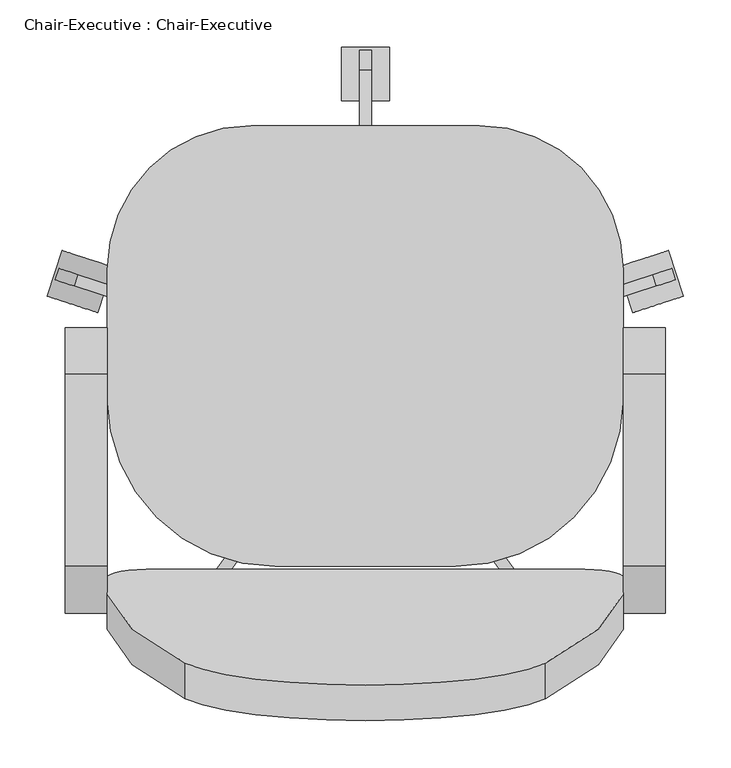
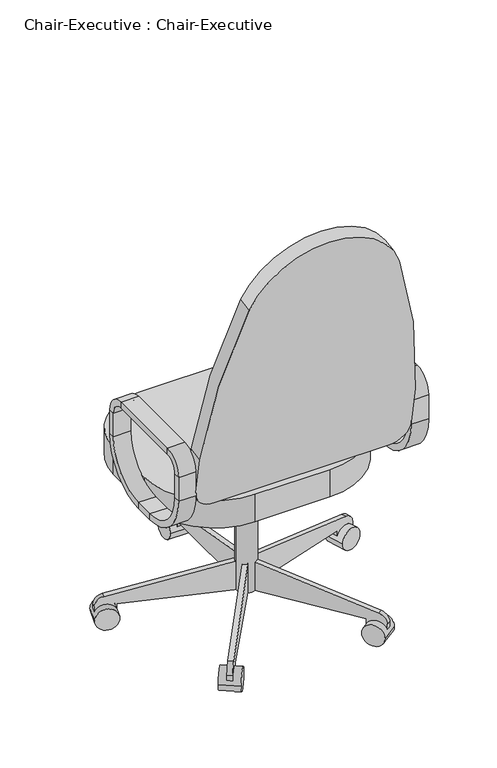
"""IFC4 building model written with IfcOpenShell, lengths in millimetres: furniture geometry, Chair-Executive : Chair-Executive."""

from ifc_helpers import new_model, si_unit, point, frame, frame_2d, origin, place, context, project, spatial, polyline, circle_curve, trimmed, segment, composite_curve, outline, extrude, source, transform, mapped, element, save
from ifc_brep_helpers import plane_surface, cylinder_surface, revolved_surface, advanced_brep


def chair_executive_chair_executive_a6d00652(model_context):
    return source(origin(), model_context, "Body", "SolidModel", [
        extrude(outline(polyline([(69.7459016, 383.7835944), (69.7459016, 371.0835944), (18.9459016, 283.0954134), (-19.1540984, 283.0954134), (-19.1540984, 383.7835944), (69.7459016, 383.7835944)])), frame((90.1908197, 0.0, 0.0), z_axis=(1.0, 0.0, 0.0), x_axis=(0.0, 1.0, 0.0)), (0.0, 0.0, 1.0), 101.6),
        extrude(outline(composite_curve([segment(polyline([(311.0459016, 53.5835944), (18.9459016, 53.5835944), (18.9459016, 129.7835944), (44.3459016, 129.7835944), (340.8565654, 77.5007643)]), True, "CONTINUOUS"), segment(trimmed(circle_curve(frame_2d((336.4459016, 52.4866474)), 25.4), [point((340.8565654, 77.5007643))], [point((361.8459016, 52.4866474))], False, "CARTESIAN"), True, "CONTINUOUS"), segment(polyline([(361.8459016, 52.4866474), (361.8459016, 28.1835944), (311.0459016, 28.1835944), (311.0459016, 53.5835944)]), True, "CONTINUOUS")], self_intersect=False)), frame((134.6408197, 0.0, 0.0), z_axis=(1.0, 0.0, 0.0), x_axis=(0.0, 1.0, 0.0)), (0.0, 0.0, 1.0), 12.7),
        extrude(outline(composite_curve([segment(trimmed(circle_curve(frame_2d((336.4459016, 28.1835944)), 28.2002727), [point((308.2456289, 28.1835944))], [point((364.6461744, 28.1835944))], False, "CARTESIAN"), True, "CONTINUOUS"), segment(trimmed(circle_curve(frame_2d((336.4459016, 28.1835944)), 28.2002727), [point((364.6461744, 28.1835944))], [point((308.2456289, 28.1835944))], False, "CARTESIAN"), True, "CONTINUOUS")], self_intersect=False)), frame((115.5908197, 0.0, 0.0), z_axis=(1.0, 0.0, 0.0), x_axis=(0.0, 1.0, 0.0)), (0.0, 0.0, 1.0), 50.8),
        extrude(outline(composite_curve([segment(polyline([(25.4, 0.0), (25.4, 292.1000001), (101.6, 292.1000001), (101.6, 266.7), (49.3171699, -29.8106636)]), True, "CONTINUOUS"), segment(trimmed(circle_curve(frame_2d((24.303053, -25.4)), 25.4), [point((49.3171699, -29.8106636))], [point((24.303053, -50.8))], False, "CARTESIAN"), True, "CONTINUOUS"), segment(polyline([(24.303053, -50.8), (0.0, -50.8), (0.0, 0.0), (25.4, 0.0)]), True, "CONTINUOUS")], self_intersect=False)), frame((-138.7750467, 103.1705568, 28.1835944), z_axis=(0.3090169943749487, 0.9510565162951532, 0.0), x_axis=(0.0, 0.0, 1.0)), (0.0, 0.0, 1.0), 12.7),
        extrude(outline(composite_curve([segment(trimmed(circle_curve(frame_2d((0.0, -28.2002727)), 28.2002727), [point((0.0, -56.4005454))], [point((0.0, 0.0))], False, "CARTESIAN"), True, "CONTINUOUS"), segment(trimmed(circle_curve(frame_2d((0.0, -28.2002727)), 28.2002727), [point((0.0, 0.0))], [point((0.0, -56.4005454))], False, "CARTESIAN"), True, "CONTINUOUS")], self_intersect=False)), frame((-195.638709, 101.6163254, 28.1835944), z_axis=(0.3090169943749487, 0.9510565162951532, 0.0), x_axis=(0.0, 0.0, -1.0)), (0.0, 0.0, 1.0), 50.8),
        extrude(outline(composite_curve([segment(polyline([(25.4, 0.0), (25.4, 292.1), (101.6, 292.1), (101.6, 266.7), (49.3171699, -29.8106637)]), True, "CONTINUOUS"), segment(trimmed(circle_curve(frame_2d((24.303053, -25.3999999)), 25.4), [point((49.3171699, -29.8106637))], [point((24.303053, -50.8))], False, "CARTESIAN"), True, "CONTINUOUS"), segment(polyline([(24.303053, -50.8), (0.0, -50.8), (0.0, 0.0), (25.4, 0.0)]), True, "CONTINUOUS")], self_intersect=False)), frame((-25.5639946, -221.1003988, 28.1835944), z_axis=(-0.8090169943749459, 0.5877852522924754, 0.0), x_axis=(0.0, 0.0, 1.0)), (0.0, 0.0, 1.0), 12.7),
        extrude(outline(composite_curve([segment(trimmed(circle_curve(frame_2d((0.0, -28.2002727)), 28.2002727), [point((0.0, -56.4005455))], [point((0.0, 0.0))], False, "CARTESIAN"), True, "CONTINUOUS"), segment(trimmed(circle_curve(frame_2d((0.0, -28.2002727)), 28.2002727), [point((0.0, 0.0))], [point((0.0, -56.4005455))], False, "CARTESIAN"), True, "CONTINUOUS")], self_intersect=False)), frame((-41.6576707, -275.6612394, 28.1835944), z_axis=(-0.8090169943749458, 0.5877852522924754, 0.0), x_axis=(0.0, 0.0, -1.0)), (0.0, 0.0, 1.0), 50.8),
        extrude(outline(composite_curve([segment(polyline([(-25.4, 0.0), (0.0, 0.0), (0.0, -50.8), (-24.303053, -50.8)]), True, "CONTINUOUS"), segment(trimmed(circle_curve(frame_2d((-24.303053, -25.3999999)), 25.4), [point((-24.303053, -50.8))], [point((-49.3171699, -29.8106636))], False, "CARTESIAN"), True, "CONTINUOUS"), segment(polyline([(-49.3171699, -29.8106636), (-101.6, 266.7), (-101.6, 292.1), (-25.4, 292.1), (-25.4, 0.0)]), True, "CONTINUOUS")], self_intersect=False)), frame((307.545634, -221.1003988, 28.1835944), z_axis=(0.8090169943749499, 0.5877852522924699, 0.0), x_axis=(0.0, 0.0, -1.0)), (0.0, 0.0, 1.0), 12.7),
        extrude(outline(composite_curve([segment(trimmed(circle_curve(frame_2d((0.0, -28.2002727)), 28.2002727), [point((0.0, -56.4005455))], [point((0.0, 0.0))], False, "CARTESIAN"), True, "CONTINUOUS"), segment(trimmed(circle_curve(frame_2d((0.0, -28.2002727)), 28.2002727), [point((0.0, 0.0))], [point((0.0, -56.4005455))], False, "CARTESIAN"), True, "CONTINUOUS")], self_intersect=False)), frame((323.63931, -275.6612394, 28.1835944), z_axis=(0.8090169943749499, 0.5877852522924699, 0.0), x_axis=(0.0, 0.0, 1.0)), (0.0, 0.0, 1.0), 50.8),
        extrude(outline(composite_curve([segment(polyline([(-25.4, 0.0), (0.0, 0.0), (0.0, -50.8), (-24.303053, -50.8)]), True, "CONTINUOUS"), segment(trimmed(circle_curve(frame_2d((-24.303053, -25.4)), 25.4), [point((-24.303053, -50.8))], [point((-49.3171699, -29.8106637))], False, "CARTESIAN"), True, "CONTINUOUS"), segment(polyline([(-49.3171699, -29.8106637), (-101.6, 266.7), (-101.6, 292.1), (-25.4, 292.1), (-25.4, 0.0)]), True, "CONTINUOUS")], self_intersect=False)), frame((420.756686, 103.1705568, 28.1835944), z_axis=(-0.3090169943749423, 0.9510565162951553, 0.0), x_axis=(0.0, 0.0, -1.0)), (0.0, 0.0, 1.0), 12.7),
        extrude(outline(composite_curve([segment(trimmed(circle_curve(frame_2d((0.0, -28.2002727)), 28.2002727), [point((0.0, -56.4005455))], [point((0.0, 0.0))], False, "CARTESIAN"), True, "CONTINUOUS"), segment(trimmed(circle_curve(frame_2d((0.0, -28.2002727)), 28.2002727), [point((0.0, 0.0))], [point((0.0, -56.4005455))], False, "CARTESIAN"), True, "CONTINUOUS")], self_intersect=False)), frame((477.6203484, 101.6163254, 28.1835944), z_axis=(-0.3090169943749423, 0.9510565162951553, 0.0), x_axis=(0.0, 0.0, 1.0)), (0.0, 0.0, 1.0), 50.8),
        extrude(outline(composite_curve([segment(trimmed(circle_curve(frame_2d((140.9908197, 18.9459016)), 25.4), [point((115.5908197, 18.9459016))], [point((166.3908197, 18.9459016))], False, "CARTESIAN"), True, "CONTINUOUS"), segment(trimmed(circle_curve(frame_2d((140.9908197, 18.9459016)), 25.4), [point((166.3908197, 18.9459016))], [point((115.5908197, 18.9459016))], False, "CARTESIAN"), True, "CONTINUOUS")], self_intersect=False)), frame((0.0, 0.0, 53.5835944), z_axis=(0.0, 0.0, 1.0), x_axis=(1.0, 0.0, 0.0)), (0.0, 0.0, 1.0), 330.5914056),
        extrude(outline(composite_curve([segment(trimmed(circle_curve(frame_2d((20.3408197, 129.4961016)), 152.4), [point((-132.0591803, 129.4961016))], [point((20.3408197, 281.8961016))], False, "CARTESIAN"), True, "CONTINUOUS"), segment(polyline([(20.3408197, 281.8961016), (261.6408197, 281.8961016)]), True, "CONTINUOUS"), segment(trimmed(circle_curve(frame_2d((261.6408197, 129.4961016)), 152.4), [point((261.6408197, 281.8961016))], [point((414.0408197, 129.4961016))], False, "CARTESIAN"), True, "CONTINUOUS"), segment(polyline([(414.0408197, 129.4961016), (414.0408197, -6.4540984)]), True, "CONTINUOUS"), segment(trimmed(circle_curve(frame_2d((236.2408197, -6.4540984)), 177.8), [point((414.0408197, -6.4540984))], [point((236.2408197, -184.2540984))], False, "CARTESIAN"), True, "CONTINUOUS"), segment(polyline([(236.2408197, -184.2540984), (45.7408197, -184.2540984)]), True, "CONTINUOUS"), segment(trimmed(circle_curve(frame_2d((45.7408197, -6.4540984)), 177.8), [point((45.7408197, -184.2540984))], [point((-132.0591803, -6.4540984))], False, "CARTESIAN"), True, "CONTINUOUS"), segment(polyline([(-132.0591803, -6.4540984), (-132.0591803, 129.4961016)]), True, "CONTINUOUS")], self_intersect=False)), frame((0.0, 0.0, 383.7835944), z_axis=(0.0, 0.0, 1.0), x_axis=(1.0, 0.0, 0.0)), (0.0, 0.0, 1.0), 73.4164056),
        extrude(outline(composite_curve([segment(trimmed(circle_curve(frame_2d((0.0, -50.8)), 50.8), [point((0.0, 0.0))], [point((50.8, -50.8))], False, "CARTESIAN"), True, "CONTINUOUS"), segment(polyline([(50.8, -50.8), (50.8, -152.4)]), True, "CONTINUOUS"), segment(trimmed(circle_curve(frame_2d((-1471.2021854, -74.3913617)), 1524.0), [point((50.8, -152.4))], [point((-31.75, -574.9444618))], False, "CARTESIAN"), True, "CONTINUOUS"), segment(trimmed(circle_curve(frame_2d((-222.25, -504.2338544)), 203.2), [point((-31.75, -574.9444618))], [point((-412.75, -574.9444618))], False, "CARTESIAN"), True, "CONTINUOUS"), segment(trimmed(circle_curve(frame_2d((1026.7021854, -74.3913617)), 1524.0), [point((-412.75, -574.9444618))], [point((-495.3, -152.4))], False, "CARTESIAN"), True, "CONTINUOUS"), segment(polyline([(-495.3, -152.4), (-495.3, -50.8)]), True, "CONTINUOUS"), segment(trimmed(circle_curve(frame_2d((-444.5, -50.8)), 50.8), [point((-495.3, -50.8))], [point((-444.5, 0.0))], False, "CARTESIAN"), True, "CONTINUOUS"), segment(polyline([(-444.5, 0.0), (0.0, 0.0)]), True, "CONTINUOUS")], self_intersect=False)), frame((363.2408197, -224.5698964, 503.1641822), z_axis=(0.0, 0.9848077530122084, 0.17364817766692853), x_axis=(1.0, 0.0, 0.0)), (0.0, 0.0, 1.0), 38.1),
        advanced_brep(
        [(414.0408197, -233.6623012, 546.1), (414.0408197, -108.0540984, 420.4917972), (458.4908197, -108.0540984, 420.4917972), (458.4908197, -233.6623012, 546.1), (414.0408197, -217.7873012, 546.1), (414.0408197, -108.0540984, 436.3667972), (458.4908197, -217.7873012, 546.1), (458.4908197, -108.0540984, 436.3667972), (458.4908197, -233.6623012, 609.6), (414.0408197, -233.6623012, 609.6), (414.0408197, -217.7873012, 609.6), (458.4908197, -217.7873012, 609.6), (414.0408197, -184.2540984, 659.0082028), (458.4908197, -184.2540984, 659.0082028), (414.0408197, -184.2540984, 643.1332028), (458.4908197, -184.2540984, 643.1332028), (458.4908197, 18.9459016, 659.0082028), (414.0408197, 18.9459016, 659.0082028), (414.0408197, 18.9459016, 643.1332028), (458.4908197, 18.9459016, 643.1332028), (414.0408197, 68.3541044, 609.6), (458.4908197, 68.3541044, 609.6), (414.0408197, 52.4791044, 609.6), (458.4908197, 52.4791044, 609.6), (458.4908197, 68.3541044, 546.1), (414.0408197, 68.3541044, 546.1), (414.0408197, 52.4791044, 546.1), (458.4908197, 52.4791044, 546.1), (414.0408197, -57.2540984, 420.4917972), (458.4908197, -57.2540984, 420.4917972), (414.0408197, -57.2540984, 436.3667972), (458.4908197, -57.2540984, 436.3667972)],
        [
            (0, 1, circle_curve(frame((414.0408197, -108.0540984, 546.1), z_axis=(1.0, 0.0, 0.0), x_axis=(0.0, 0.0, -1.0)), 125.6082028)),
            (1, 2),
            (2, 3, circle_curve(frame((458.4908197, -108.0540984, 546.1), z_axis=(-1.0, 0.0, 0.0), x_axis=(0.0, 0.0, -1.0)), 125.6082028)),
            (3, 0),
            (4, 5, circle_curve(frame((414.0408197, -108.0540984, 546.1), z_axis=(1.0, 0.0, 0.0), x_axis=(0.0, 0.0, -1.0)), 109.7332028)),
            (5, 1),
            (0, 4),
            (6, 7, circle_curve(frame((458.4908197, -108.0540984, 546.1), z_axis=(1.0, 0.0, 0.0), x_axis=(0.0, 0.0, -1.0)), 109.7332028)),
            (7, 5),
            (4, 6),
            (2, 7),
            (6, 3),
            (3, 8),
            (8, 9),
            (9, 0),
            (9, 10),
            (10, 4),
            (10, 11),
            (11, 6),
            (11, 8),
            (12, 9, circle_curve(frame((414.0408197, -184.2540984, 609.6), z_axis=(1.0, 0.0, 0.0), x_axis=(0.0, -1.0, 0.0)), 49.4082028)),
            (8, 13, circle_curve(frame((458.4908197, -184.2540984, 609.6), z_axis=(-1.0, 0.0, 0.0), x_axis=(0.0, -1.0, 0.0)), 49.4082028)),
            (13, 12),
            (14, 10, circle_curve(frame((414.0408197, -184.2540984, 609.6), z_axis=(1.0, 0.0, 0.0), x_axis=(0.0, -1.0, 0.0)), 33.5332028)),
            (12, 14),
            (15, 11, circle_curve(frame((458.4908197, -184.2540984, 609.6), z_axis=(1.0, 0.0, 0.0), x_axis=(0.0, -1.0, 0.0)), 33.5332028)),
            (14, 15),
            (15, 13),
            (13, 16),
            (16, 17),
            (17, 12),
            (17, 18),
            (18, 14),
            (18, 19),
            (19, 15),
            (19, 16),
            (20, 17, circle_curve(frame((414.0408197, 18.9459016, 609.6), z_axis=(1.0, 0.0, 0.0), x_axis=(0.0, 0.0, 1.0)), 49.4082028)),
            (16, 21, circle_curve(frame((458.4908197, 18.9459016, 609.6), z_axis=(-1.0, 0.0, 0.0), x_axis=(0.0, 0.0, 1.0)), 49.4082028)),
            (21, 20),
            (22, 18, circle_curve(frame((414.0408197, 18.9459016, 609.6), z_axis=(1.0, 0.0, 0.0), x_axis=(0.0, 0.0, 1.0)), 33.5332028)),
            (20, 22),
            (23, 19, circle_curve(frame((458.4908197, 18.9459016, 609.6), z_axis=(1.0, 0.0, 0.0), x_axis=(0.0, 0.0, 1.0)), 33.5332028)),
            (22, 23),
            (23, 21),
            (21, 24),
            (24, 25),
            (25, 20),
            (25, 26),
            (26, 22),
            (26, 27),
            (27, 23),
            (27, 24),
            (28, 25, circle_curve(frame((414.0408197, -57.2540984, 546.1), z_axis=(1.0, 0.0, 0.0), x_axis=(0.0, 1.0, 0.0)), 125.6082028)),
            (24, 29, circle_curve(frame((458.4908197, -57.2540984, 546.1), z_axis=(-1.0, 0.0, 0.0), x_axis=(0.0, 1.0, 0.0)), 125.6082028)),
            (29, 28),
            (30, 26, circle_curve(frame((414.0408197, -57.2540984, 546.1), z_axis=(1.0, 0.0, 0.0), x_axis=(0.0, 1.0, 0.0)), 109.7332028)),
            (28, 30),
            (31, 27, circle_curve(frame((458.4908197, -57.2540984, 546.1), z_axis=(1.0, 0.0, 0.0), x_axis=(0.0, 1.0, 0.0)), 109.7332028)),
            (30, 31),
            (31, 29),
            (29, 2),
            (1, 28),
            (5, 30),
            (7, 31),
        ],
        [
            cylinder_surface(frame((414.0408197, -108.0540984, 546.1), z_axis=(-1.0, 0.0, 0.0), x_axis=(0.0, 0.0, -1.0)), 125.6082028),
            plane_surface(frame((414.0408197, -108.0540984, 546.1), z_axis=(-1.0, 0.0, 0.0), x_axis=(0.0, 0.0, -1.0))),
            revolved_surface(polyline([(414.0408197, -108.0540984, 436.3667972), (458.4908197, -108.0540984, 436.3667972)]), (414.0408197, -108.0540984, 546.1), (-1.0, 0.0, 0.0)),
            plane_surface(frame((458.4908197, -108.0540984, 546.1), z_axis=(1.0, 0.0, 0.0), x_axis=(0.0, 0.0, -1.0))),
            plane_surface(frame((458.4908197, -233.6623012, 546.1), z_axis=(0.0, -1.0, 0.0), x_axis=(0.0, 0.0, 1.0))),
            plane_surface(frame((414.0408197, -233.6623012, 546.1), z_axis=(-1.0, 0.0, 0.0), x_axis=(0.0, 0.0, 1.0))),
            plane_surface(frame((414.0408197, -217.7873012, 546.1), z_axis=(0.0, 1.0, 0.0), x_axis=(0.0, 0.0, 1.0))),
            plane_surface(frame((458.4908197, -217.7873012, 546.1), z_axis=(1.0, 0.0, 0.0), x_axis=(0.0, 0.0, 1.0))),
            cylinder_surface(frame((414.0408197, -184.2540984, 609.6), z_axis=(-1.0, 0.0, 0.0), x_axis=(0.0, -1.0, 0.0)), 49.4082028),
            plane_surface(frame((414.0408197, -184.2540984, 609.6), z_axis=(-1.0, 0.0, 0.0), x_axis=(0.0, -1.0, 0.0))),
            revolved_surface(polyline([(414.0408197, -217.7873012, 609.6), (458.4908197, -217.7873012, 609.6)]), (414.0408197, -184.2540984, 609.6), (-1.0, 0.0, 0.0)),
            plane_surface(frame((458.4908197, -184.2540984, 609.6), z_axis=(1.0, 0.0, 0.0), x_axis=(0.0, -1.0, 0.0))),
            plane_surface(frame((458.4908197, -184.2540984, 659.0082028), z_axis=(0.0, 0.0, 1.0), x_axis=(0.0, 1.0, 0.0))),
            plane_surface(frame((414.0408197, -184.2540984, 659.0082028), z_axis=(-1.0, 0.0, 0.0), x_axis=(0.0, 1.0, 0.0))),
            plane_surface(frame((414.0408197, -184.2540984, 643.1332028), z_axis=(0.0, 0.0, -1.0), x_axis=(0.0, 1.0, 0.0))),
            plane_surface(frame((458.4908197, -184.2540984, 643.1332028), z_axis=(1.0, 0.0, 0.0), x_axis=(0.0, 1.0, 0.0))),
            cylinder_surface(frame((414.0408197, 18.9459016, 609.6), z_axis=(-1.0, 0.0, 0.0), x_axis=(0.0, 0.0, 1.0)), 49.4082028),
            plane_surface(frame((414.0408197, 18.9459016, 609.6), z_axis=(-1.0, 0.0, 0.0), x_axis=(0.0, 0.0, 1.0))),
            revolved_surface(polyline([(414.0408197, 18.9459016, 643.1332028), (458.4908197, 18.9459016, 643.1332028)]), (414.0408197, 18.9459016, 609.6), (-1.0, 0.0, 0.0)),
            plane_surface(frame((458.4908197, 18.9459016, 609.6), z_axis=(1.0, 0.0, 0.0), x_axis=(0.0, 0.0, 1.0))),
            plane_surface(frame((458.4908197, 68.3541044, 609.6), z_axis=(0.0, 1.0, 0.0), x_axis=(0.0, 0.0, -1.0))),
            plane_surface(frame((414.0408197, 68.3541044, 609.6), z_axis=(-1.0, 0.0, 0.0), x_axis=(0.0, 0.0, -1.0))),
            plane_surface(frame((414.0408197, 52.4791044, 609.6), z_axis=(0.0, -1.0, 0.0), x_axis=(0.0, 0.0, -1.0))),
            plane_surface(frame((458.4908197, 52.4791044, 609.6), z_axis=(1.0, 0.0, 0.0), x_axis=(0.0, 0.0, -1.0))),
            cylinder_surface(frame((414.0408197, -57.2540984, 546.1), z_axis=(-1.0, 0.0, 0.0), x_axis=(0.0, 1.0, 0.0)), 125.6082028),
            plane_surface(frame((414.0408197, -57.2540984, 546.1), z_axis=(-1.0, 0.0, 0.0), x_axis=(0.0, 1.0, 0.0))),
            revolved_surface(polyline([(414.0408197, 52.479104400000004, 546.1), (458.4908197, 52.479104400000004, 546.1)]), (414.0408197, -57.2540984, 546.1), (-1.0, 0.0, 0.0)),
            plane_surface(frame((458.4908197, -57.2540984, 546.1), z_axis=(1.0, 0.0, 0.0), x_axis=(0.0, 1.0, 0.0))),
            plane_surface(frame((458.4908197, -57.2540984, 420.4917972), z_axis=(0.0, 0.0, -1.0), x_axis=(0.0, -1.0, 0.0))),
            plane_surface(frame((414.0408197, -57.2540984, 420.4917972), z_axis=(-1.0, 0.0, 0.0), x_axis=(0.0, -1.0, 0.0))),
            plane_surface(frame((414.0408197, -57.2540984, 436.3667972), z_axis=(0.0, 0.0, 1.0), x_axis=(0.0, -1.0, 0.0))),
            plane_surface(frame((458.4908197, -57.2540984, 436.3667972), z_axis=(1.0, 0.0, 0.0), x_axis=(0.0, -1.0, 0.0))),
        ],
        [
            (0, [[1, 2, 3, 4]]),
            (1, [[5, 6, -1, 7]]),
            (2, [[8, 9, -5, 10]]),
            (3, [[-3, 11, -8, 12]]),
            (4, [[-4, 13, 14, 15]]),
            (5, [[-7, -15, 16, 17]]),
            (6, [[-10, -17, 18, 19]]),
            (7, [[-12, -19, 20, -13]]),
            (8, [[21, -14, 22, 23]]),
            (9, [[24, -16, -21, 25]]),
            (10, [[26, -18, -24, 27]]),
            (11, [[-22, -20, -26, 28]]),
            (12, [[-23, 29, 30, 31]]),
            (13, [[-25, -31, 32, 33]]),
            (14, [[-27, -33, 34, 35]]),
            (15, [[-28, -35, 36, -29]]),
            (16, [[37, -30, 38, 39]]),
            (17, [[40, -32, -37, 41]]),
            (18, [[42, -34, -40, 43]]),
            (19, [[-38, -36, -42, 44]]),
            (20, [[-39, 45, 46, 47]]),
            (21, [[-41, -47, 48, 49]]),
            (22, [[-43, -49, 50, 51]]),
            (23, [[-44, -51, 52, -45]]),
            (24, [[53, -46, 54, 55]]),
            (25, [[56, -48, -53, 57]]),
            (26, [[58, -50, -56, 59]]),
            (27, [[-54, -52, -58, 60]]),
            (28, [[-55, 61, -2, 62]]),
            (29, [[-57, -62, -6, 63]]),
            (30, [[-59, -63, -9, 64]]),
            (31, [[-60, -64, -11, -61]]),
        ],
    ),
        advanced_brep(
        [(-176.5091803, -217.7873012, 546.1), (-176.5091803, -108.0540984, 436.3667972), (-176.5091803, -108.0540984, 420.4917972), (-176.5091803, -233.6623012, 546.1), (-132.0591803, -217.7873012, 546.1), (-132.0591803, -108.0540984, 436.3667972), (-132.0591803, -233.6623012, 546.1), (-132.0591803, -108.0540984, 420.4917972), (-176.5091803, -233.6623012, 609.6), (-176.5091803, -217.7873012, 609.6), (-132.0591803, -217.7873012, 609.6), (-132.0591803, -233.6623012, 609.6), (-176.5091803, -184.2540984, 643.1332028), (-176.5091803, -184.2540984, 659.0082028), (-132.0591803, -184.2540984, 643.1332028), (-132.0591803, -184.2540984, 659.0082028), (-176.5091803, 18.9459016, 659.0082028), (-176.5091803, 18.9459016, 643.1332028), (-132.0591803, 18.9459016, 643.1332028), (-132.0591803, 18.9459016, 659.0082028), (-176.5091803, 52.4791044, 609.6), (-176.5091803, 68.3541044, 609.6), (-132.0591803, 52.4791044, 609.6), (-132.0591803, 68.3541044, 609.6), (-176.5091803, 68.3541044, 546.1), (-176.5091803, 52.4791044, 546.1), (-132.0591803, 52.4791044, 546.1), (-132.0591803, 68.3541044, 546.1), (-176.5091803, -57.2540984, 436.3667972), (-176.5091803, -57.2540984, 420.4917972), (-132.0591803, -57.2540984, 436.3667972), (-132.0591803, -57.2540984, 420.4917972)],
        [
            (0, 1, circle_curve(frame((-176.5091803, -108.0540984, 546.1), z_axis=(1.0, 0.0, 0.0), x_axis=(0.0, 0.0, -1.0)), 109.7332028)),
            (1, 2),
            (2, 3, circle_curve(frame((-176.5091803, -108.0540984, 546.1), z_axis=(-1.0, 0.0, 0.0), x_axis=(0.0, 0.0, -1.0)), 125.6082028)),
            (3, 0),
            (4, 5, circle_curve(frame((-132.0591803, -108.0540984, 546.1), z_axis=(1.0, 0.0, 0.0), x_axis=(0.0, 0.0, -1.0)), 109.7332028)),
            (5, 1),
            (0, 4),
            (6, 7, circle_curve(frame((-132.0591803, -108.0540984, 546.1), z_axis=(1.0, 0.0, 0.0), x_axis=(0.0, 0.0, -1.0)), 125.6082028)),
            (7, 5),
            (4, 6),
            (2, 7),
            (6, 3),
            (3, 8),
            (8, 9),
            (9, 0),
            (9, 10),
            (10, 4),
            (10, 11),
            (11, 6),
            (11, 8),
            (12, 9, circle_curve(frame((-176.5091803, -184.2540984, 609.6), z_axis=(1.0, 0.0, 0.0), x_axis=(0.0, -1.0, 0.0)), 33.5332028)),
            (8, 13, circle_curve(frame((-176.5091803, -184.2540984, 609.6), z_axis=(-1.0, 0.0, 0.0), x_axis=(0.0, -1.0, 0.0)), 49.4082028)),
            (13, 12),
            (14, 10, circle_curve(frame((-132.0591803, -184.2540984, 609.6), z_axis=(1.0, 0.0, 0.0), x_axis=(0.0, -1.0, 0.0)), 33.5332028)),
            (12, 14),
            (15, 11, circle_curve(frame((-132.0591803, -184.2540984, 609.6), z_axis=(1.0, 0.0, 0.0), x_axis=(0.0, -1.0, 0.0)), 49.4082028)),
            (14, 15),
            (15, 13),
            (13, 16),
            (16, 17),
            (17, 12),
            (17, 18),
            (18, 14),
            (18, 19),
            (19, 15),
            (19, 16),
            (20, 17, circle_curve(frame((-176.5091803, 18.9459016, 609.6), z_axis=(1.0, 0.0, 0.0), x_axis=(0.0, 0.0, 1.0)), 33.5332028)),
            (16, 21, circle_curve(frame((-176.5091803, 18.9459016, 609.6), z_axis=(-1.0, 0.0, 0.0), x_axis=(0.0, 0.0, 1.0)), 49.4082028)),
            (21, 20),
            (22, 18, circle_curve(frame((-132.0591803, 18.9459016, 609.6), z_axis=(1.0, 0.0, 0.0), x_axis=(0.0, 0.0, 1.0)), 33.5332028)),
            (20, 22),
            (23, 19, circle_curve(frame((-132.0591803, 18.9459016, 609.6), z_axis=(1.0, 0.0, 0.0), x_axis=(0.0, 0.0, 1.0)), 49.4082028)),
            (22, 23),
            (23, 21),
            (21, 24),
            (24, 25),
            (25, 20),
            (25, 26),
            (26, 22),
            (26, 27),
            (27, 23),
            (27, 24),
            (28, 25, circle_curve(frame((-176.5091803, -57.2540984, 546.1), z_axis=(1.0, 0.0, 0.0), x_axis=(0.0, 1.0, 0.0)), 109.7332028)),
            (24, 29, circle_curve(frame((-176.5091803, -57.2540984, 546.1), z_axis=(-1.0, 0.0, 0.0), x_axis=(0.0, 1.0, 0.0)), 125.6082028)),
            (29, 28),
            (30, 26, circle_curve(frame((-132.0591803, -57.2540984, 546.1), z_axis=(1.0, 0.0, 0.0), x_axis=(0.0, 1.0, 0.0)), 109.7332028)),
            (28, 30),
            (31, 27, circle_curve(frame((-132.0591803, -57.2540984, 546.1), z_axis=(1.0, 0.0, 0.0), x_axis=(0.0, 1.0, 0.0)), 125.6082028)),
            (30, 31),
            (31, 29),
            (29, 2),
            (1, 28),
            (5, 30),
            (7, 31),
        ],
        [
            plane_surface(frame((-176.5091803, -108.0540984, 546.1), z_axis=(-1.0, 0.0, 0.0), x_axis=(0.0, 0.0, -1.0))),
            revolved_surface(polyline([(-176.5091803, -108.0540984, 436.3667972), (-132.0591803, -108.0540984, 436.3667972)]), (-132.0591803, -108.0540984, 546.1), (-1.0, 0.0, 0.0)),
            plane_surface(frame((-132.0591803, -108.0540984, 546.1), z_axis=(1.0, 0.0, 0.0), x_axis=(0.0, 0.0, -1.0))),
            cylinder_surface(frame((-132.0591803, -108.0540984, 546.1), z_axis=(-1.0, 0.0, 0.0), x_axis=(0.0, 0.0, -1.0)), 125.6082028),
            plane_surface(frame((-176.5091803, -233.6623012, 546.1), z_axis=(-1.0, 0.0, 0.0), x_axis=(0.0, 0.0, 1.0))),
            plane_surface(frame((-176.5091803, -217.7873012, 546.1), z_axis=(0.0, 1.0, 0.0), x_axis=(0.0, 0.0, 1.0))),
            plane_surface(frame((-132.0591803, -217.7873012, 546.1), z_axis=(1.0, 0.0, 0.0), x_axis=(0.0, 0.0, 1.0))),
            plane_surface(frame((-132.0591803, -233.6623012, 546.1), z_axis=(0.0, -1.0, 0.0), x_axis=(0.0, 0.0, 1.0))),
            plane_surface(frame((-176.5091803, -184.2540984, 609.6), z_axis=(-1.0, 0.0, 0.0), x_axis=(0.0, -1.0, 0.0))),
            revolved_surface(polyline([(-176.5091803, -217.7873012, 609.6), (-132.0591803, -217.7873012, 609.6)]), (-132.0591803, -184.2540984, 609.6), (-1.0, 0.0, 0.0)),
            plane_surface(frame((-132.0591803, -184.2540984, 609.6), z_axis=(1.0, 0.0, 0.0), x_axis=(0.0, -1.0, 0.0))),
            cylinder_surface(frame((-132.0591803, -184.2540984, 609.6), z_axis=(-1.0, 0.0, 0.0), x_axis=(0.0, -1.0, 0.0)), 49.4082028),
            plane_surface(frame((-176.5091803, -184.2540984, 659.0082028), z_axis=(-1.0, 0.0, 0.0), x_axis=(0.0, 1.0, 0.0))),
            plane_surface(frame((-176.5091803, -184.2540984, 643.1332028), z_axis=(0.0, 0.0, -1.0), x_axis=(0.0, 1.0, 0.0))),
            plane_surface(frame((-132.0591803, -184.2540984, 643.1332028), z_axis=(1.0, 0.0, 0.0), x_axis=(0.0, 1.0, 0.0))),
            plane_surface(frame((-132.0591803, -184.2540984, 659.0082028), z_axis=(0.0, 0.0, 1.0), x_axis=(0.0, 1.0, 0.0))),
            plane_surface(frame((-176.5091803, 18.9459016, 609.6), z_axis=(-1.0, 0.0, 0.0), x_axis=(0.0, 0.0, 1.0))),
            revolved_surface(polyline([(-176.5091803, 18.9459016, 643.1332028), (-132.0591803, 18.9459016, 643.1332028)]), (-132.0591803, 18.9459016, 609.6), (-1.0, 0.0, 0.0)),
            plane_surface(frame((-132.0591803, 18.9459016, 609.6), z_axis=(1.0, 0.0, 0.0), x_axis=(0.0, 0.0, 1.0))),
            cylinder_surface(frame((-132.0591803, 18.9459016, 609.6), z_axis=(-1.0, 0.0, 0.0), x_axis=(0.0, 0.0, 1.0)), 49.4082028),
            plane_surface(frame((-176.5091803, 68.3541044, 609.6), z_axis=(-1.0, 0.0, 0.0), x_axis=(0.0, 0.0, -1.0))),
            plane_surface(frame((-176.5091803, 52.4791044, 609.6), z_axis=(0.0, -1.0, 0.0), x_axis=(0.0, 0.0, -1.0))),
            plane_surface(frame((-132.0591803, 52.4791044, 609.6), z_axis=(1.0, 0.0, 0.0), x_axis=(0.0, 0.0, -1.0))),
            plane_surface(frame((-132.0591803, 68.3541044, 609.6), z_axis=(0.0, 1.0, 0.0), x_axis=(0.0, 0.0, -1.0))),
            plane_surface(frame((-176.5091803, -57.2540984, 546.1), z_axis=(-1.0, 0.0, 0.0), x_axis=(0.0, 1.0, 0.0))),
            revolved_surface(polyline([(-176.5091803, 52.479104400000004, 546.1), (-132.0591803, 52.479104400000004, 546.1)]), (-132.0591803, -57.2540984, 546.1), (-1.0, 0.0, 0.0)),
            plane_surface(frame((-132.0591803, -57.2540984, 546.1), z_axis=(1.0, 0.0, 0.0), x_axis=(0.0, 1.0, 0.0))),
            cylinder_surface(frame((-132.0591803, -57.2540984, 546.1), z_axis=(-1.0, 0.0, 0.0), x_axis=(0.0, 1.0, 0.0)), 125.6082028),
            plane_surface(frame((-176.5091803, -57.2540984, 420.4917972), z_axis=(-1.0, 0.0, 0.0), x_axis=(0.0, -1.0, 0.0))),
            plane_surface(frame((-176.5091803, -57.2540984, 436.3667972), z_axis=(0.0, 0.0, 1.0), x_axis=(0.0, -1.0, 0.0))),
            plane_surface(frame((-132.0591803, -57.2540984, 436.3667972), z_axis=(1.0, 0.0, 0.0), x_axis=(0.0, -1.0, 0.0))),
            plane_surface(frame((-132.0591803, -57.2540984, 420.4917972), z_axis=(0.0, 0.0, -1.0), x_axis=(0.0, -1.0, 0.0))),
        ],
        [
            (0, [[1, 2, 3, 4]]),
            (1, [[5, 6, -1, 7]]),
            (2, [[8, 9, -5, 10]]),
            (3, [[-3, 11, -8, 12]]),
            (4, [[-4, 13, 14, 15]]),
            (5, [[-7, -15, 16, 17]]),
            (6, [[-10, -17, 18, 19]]),
            (7, [[-12, -19, 20, -13]]),
            (8, [[21, -14, 22, 23]]),
            (9, [[24, -16, -21, 25]]),
            (10, [[26, -18, -24, 27]]),
            (11, [[-22, -20, -26, 28]]),
            (12, [[-23, 29, 30, 31]]),
            (13, [[-25, -31, 32, 33]]),
            (14, [[-27, -33, 34, 35]]),
            (15, [[-28, -35, 36, -29]]),
            (16, [[37, -30, 38, 39]]),
            (17, [[40, -32, -37, 41]]),
            (18, [[42, -34, -40, 43]]),
            (19, [[-38, -36, -42, 44]]),
            (20, [[-39, 45, 46, 47]]),
            (21, [[-41, -47, 48, 49]]),
            (22, [[-43, -49, 50, 51]]),
            (23, [[-44, -51, 52, -45]]),
            (24, [[53, -46, 54, 55]]),
            (25, [[56, -48, -53, 57]]),
            (26, [[58, -50, -56, 59]]),
            (27, [[-54, -52, -58, 60]]),
            (28, [[-55, 61, -2, 62]]),
            (29, [[-57, -62, -6, 63]]),
            (30, [[-59, -63, -9, 64]]),
            (31, [[-60, -64, -11, -61]]),
        ],
    ),
    ])


if __name__ == "__main__":
    model = new_model("IFC4")
    model_context = context("Model", 3, world=origin())
    ifc_project = project(units=[si_unit("LENGTHUNIT", "METRE", prefix="MILLI")], contexts=[model_context])
    site = spatial("IfcSite", under=ifc_project)
    building = spatial("IfcBuilding", under=site)
    placement = place(None, origin())
    chair_executive_chair_executive_shape = chair_executive_chair_executive_a6d00652(model_context)
    element("IfcFurniture", 1, ObjectType="Chair-Executive : Chair-Executive", at=placement, inside=building, context=model_context, shape_type="MappedRepresentation", body=[
        mapped(chair_executive_chair_executive_shape, transform((0.0, 0.0, 0.0), x_axis=(1.0, 0.0, 0.0), y_axis=(0.0, 1.0, 0.0), z_axis=(0.0, 0.0, 1.0))),
    ])
    save(model, "model.ifc")

# Revit data of these elements
# Type "Chair-Executive : Chair-Executive"
#   Assembly Code = "E2020200"
#   Base/Arms Material = Plastic, Opaque Black
#   Casters Material = Plastic, Opaque Black
#   Seat/Back Material = Textile - Slate Blue
#   Default Elevation = 0
# Element 1 (IfcFurniture, "Chair-Executive : Chair-Executive")
#   Materials on its faces: "Plastic, Opaque Black", "Textile - Slate Blue"
# Materials
#   "Plastic, Opaque Black": class "Plastic", colour RGB 0 0 0, transparency 0, Description = "Plastic, generic, opaque black", Cost = 0
#   "Textile - Slate Blue": class "Fabric", colour RGB 98 102 118, transparency 0
